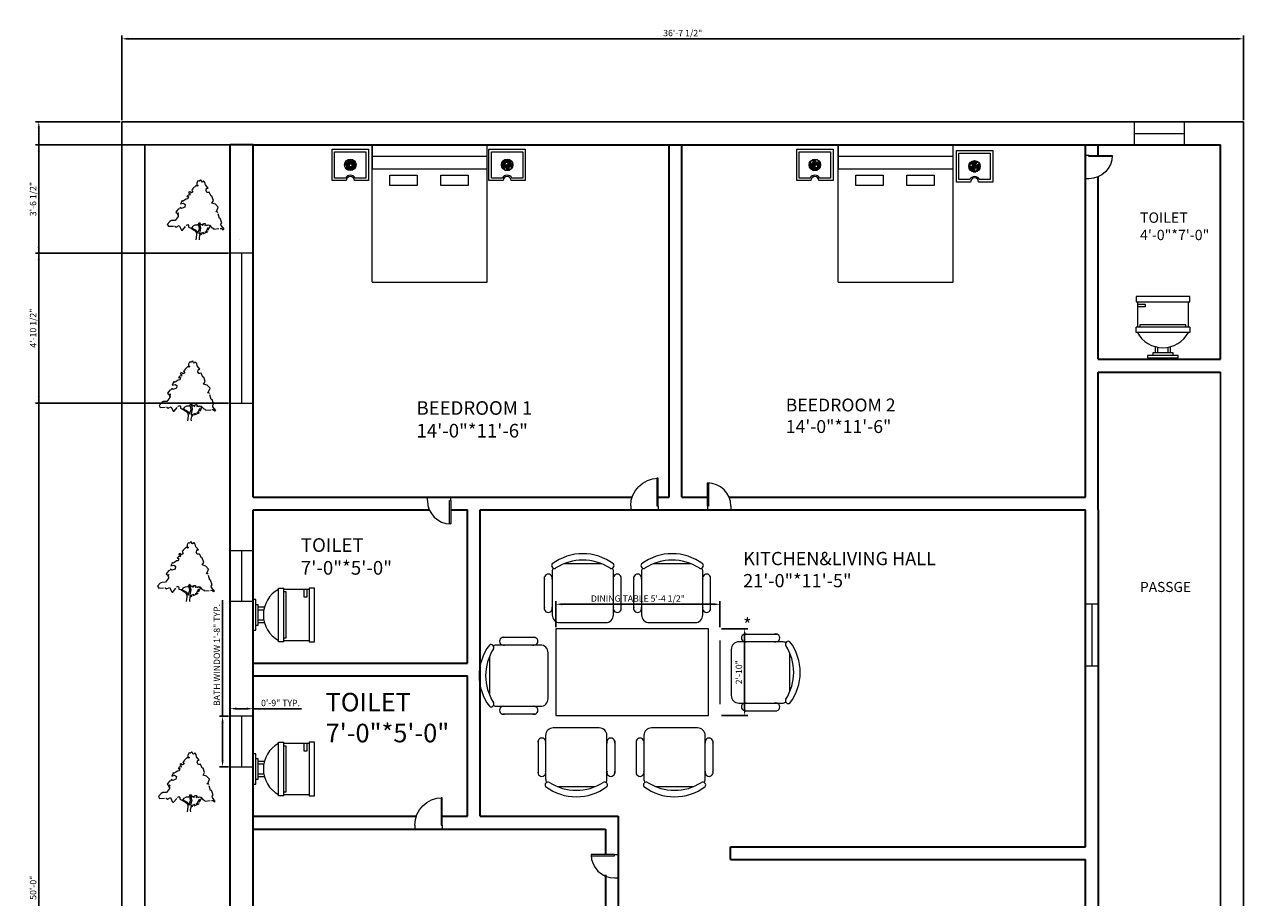
# Model space of a CAD drawing. Units: inches. Extents: x 2432 to 3786, y 1221 to 1905.
# Tile 2 of 4: x 2432 to 2910, y 1563 to 1905. Entities that reach past the tile are written whole.
import ezdxf

# ---------------------------------------------------------------- set-up
doc = ezdxf.new("R2010")
doc.units = ezdxf.units.IN
doc.linetypes.add('ACAD_ISO02W100', pattern=[15, 12, -3])
for name, color, linetype, lineweight, true_color in [('A-ANNO-DIMS', 32, 'Continuous', 18, 0xcd6928), ('A-AREA-IDEN', 244, 'Continuous', 18, 0x991b1e), ('A-FURN', 32, 'Continuous', 13, 0xcd6928), ('A-GLAZ', 116, 'Continuous', 18, 0x136734), ('A-WALL', 67, 'Continuous', 35, 0x727430), ('C-PROP', 67, 'Continuous', 25, 0x727430)]:
    doc.layers.add(name, color=color, linetype=linetype, lineweight=lineweight, true_color=true_color)
for name, color, linetype, lineweight in [('A-DOOR', 4, 'Continuous', 18), ('A-FLOR-FIXT', 9, 'Continuous', 18), ('L-PLNT', 3, 'ACAD_ISO02W100', 13)]:
    doc.layers.add(name, color=color, linetype=linetype, lineweight=lineweight)
doc.styles.get("Standard").update_dxf_attribs({"font": 'arial.ttf'})
doc.dimstyles.new('ISO-25', dxfattribs={"dimtxt": 2.5, "dimasz": 2.5, "dimexe": 1.25, "dimexo": 0.625, "dimtad": 1, "dimdec": 3, "dimlunit": 4, "dimtxsty": 'Standard', "dimcen": 2.5, "dimadec": 0, "dimazin": 0, "dimtfac": 1, "dimtdec": 3, "dimtmove": 0, "dimatfit": 3, "dimfxl": 1, "dimarcsym": 0})

# ---------------------------------------------------------------- blocks, each defined once
blk = doc.blocks.new('*U4')
for points in [[(22.0124, 137.721), (18.5475, 141.5624), (15.5282, 138.2446), (13.8028, 139.3505), (13.3714, 142.1153), (11.2148, 143.2214), (8.1954, 140.4564), (4.7447, 141.0094), (2.1567, 136.0326), (2.1567, 131.6088), (5.6074, 129.9499), (3.0193, 128.2909), (0.4313, 130.5029), (-6.9015, 123.3141), (-6.9015, 121.6552), (-9.9208, 119.9963), (-9.0581, 118.3373), (-6.9015, 115.0195), (-10.7835, 112.2546), (-14.6656, 115.0195), (-16.8222, 114.4665), (-17.6849, 112.2546), (-14.6656, 111.7016), (-14.2342, 107.2778), (-17.6065, 107.8307), (-21.5669, 103.9599), (-17.2536, 103.4069), (-18.9789, 97.8771), (-22.8609, 97.3241), (-27.1743, 94.5593), (-32.3504, 91.7944), (-32.7817, 94.0063), (-36.6638, 85.7116), (-29.7624, 87.3705), (-25.449, 84.6056), (-26.743, 77.9699), (-34.507, 75.205), (-37.9578, 77.4169), (-39.2518, 74.099), (-42.2711, 73.5461), (-44.8592, 70.2282), (-47.8786, 66.3574), (-43.9965, 63.0395), (-41.4085, 64.6985), (-44.3346, 59.8898), (-42.2089, 60.1377), (-42.5159, 55.7849), (-49.6039, 46.4502), (-58.2307, 45.8972), (-62.1127, 43.6853), (-68.5828, 36.4966), (-65.9947, 32.0727), (-50.0352, 32.6257), (-47.0159, 30.4138), (-39.6831, 33.7317), (-34.507, 22.6721), (-32.3504, 22.6721), (-22.4296, 34.8376), (-19.4102, 36.4966), (-17.2536, 33.7317), (-17.2536, 29.8608), (-13.8028, 28.7549), (-9.0581, 28.7549), (-7.3328, 32.6257), (-1.7254, 35.3906), (3.8821, 35.9436), (6.4701, 38.1555), (6.9014, 38.7085), (8.1954, 41.4734), (9.9208, 40.3674), (11.2148, 35.9436), (14.2341, 37.6025), (15.0968, 36.4966), (15.9595, 33.7317), (18.9789, 38.7085), (21.9982, 38.7085), (23.2922, 36.4966), (21.9982, 34.2847), (25.4489, 35.3906), (26.743, 33.7317), (29.7623, 35.9436), (32.7817, 34.8376), (38.8204, 28.7549), (41.4084, 27.6489), (43.5651, 25.437), (61.6813, 27.0959), (65.132, 23.7781), (67.7201, 24.884), (60.8186, 33.7317), (60.3873, 37.0495), (62.544, 40.3674), (58.662, 50.874), (56.5053, 50.874), (52.1919, 66.3574), (47.8785, 66.9103), (50.4665, 69.1222), (53.9172, 77.9699), (47.0158, 85.1586), (38.3891, 87.9235), (42.2711, 94.0063)], [(42.2711, 94.0063), (38.8204, 104.5129), (36.6637, 104.5129), (32.3503, 113.9135), (29.7623, 113.3605), (26.743, 113.3605), (24.5862, 117.7844), (25.8802, 123.8671), (29.331, 123.8671), (22.8609, 131.6088), (21.9982, 137.6916)], [(-9.9208, 28.2019), (0, 23.2251), (3.4507, 19.9072), (4.7447, 15.4834), (8.6267, 27.0959), (6.4701, 37.6025)], [(34.5071, 33.1787), (27.1743, 18.2483), (9.0581, 10.5066), (7.7641, 3.8708), (8.1954, 0)], [(8.1954, 40.3674), (11.2148, 27.6489), (8.1954, 13.8245), (24.5862, 19.9072), (32.7817, 34.2847)], [(-12.9401, 28.7549), (-2.588, 22.1191), (0.8626, 17.6953), (1.7253, 11.6125), (0, 0)]]:
    blk.add_lwpolyline(points)
blk = doc.blocks.new('FC15X27A')
for p, q in [((7.53125, 0), (-7.53125, 0)), ((-7.53125, 0), (-7.53125, -26.5)), ((7.53125, -26.5), (7.53125, 0)), ((-7.53125, -26.5), (7.53125, -26.5)), ((-5.53125, -28.5), (5.53125, -28.5))]:
    blk.add_line(p, q)
blk = doc.blocks.new('CHAIR7')
for p, q in [((5.12, 15.04), (17.88, 15.04)), ((20, 12), (3, 12)), ((0, 9), (0, -9)), ((23, -7.44), (23, 7.44)), ((3, -12), (20, -12)), ((5.12, -15), (17.88, -15))]:
    blk.add_line(p, q)
for centre, radius, start, end in [((5.56, 13.54), 1.56, 73.7398, 286.2602), ((17.44, 13.54), 1.56, 253.7398, 106.2602), ((3, 9), 3, 90, 180), ((20, 9), 3, 62.4156, 90), ((22.34, 11.12), 1.1, 53.3099, 212.0274), ((4.82, 0), 19.64, 327.5758, 32.4242), ((7, 0), 20, 323.1301, 36.8699), ((3, -9), 3, 180, 270), ((5.56, -13.5), 1.56, 73.7398, 286.2602), ((17.44, -13.5), 1.56, 253.7398, 106.2602), ((20, -9), 3, 270, 297.5844), ((22.34, -11.12), 1.1, 147.9726, 306.6901)]:
    blk.add_arc(centre, radius, start, end)
blk = doc.blocks.new('*U9')
for p, q in [((0, 0), (0, -6)), ((40, 0), (40, -6))]:
    blk.add_line(p, q)
blk.add_lwpolyline([(0, 0), (0, 40), (1.75, 40), (1.75, 0)], close=True)
blk.add_arc((0, 0), 40, 0, 90)
blk = doc.blocks.new('*U10')
for p, q in [((0, 0), (0, -6)), ((-40, 0), (-40, -6))]:
    blk.add_line(p, q)
blk.add_lwpolyline([(0, 0), (0, 40), (-1.75, 40), (-1.75, 0)], close=True)
blk.add_arc((0, 0), 40, 90, 180)
blk = doc.blocks.new('*U12')
for p, q in [((-10, 22), (-10, 12)), ((-10, 21), (-7, 21)), ((-7, 20), (-10, 20)), ((-7, 21), (-7, 20)), ((10, 12), (10, 22)), ((10.5, 12), (-10.5, 12)), ((-10.5, 10), (-10.5, 12)), ((10.5, 10), (-10.5, 10)), ((9, 13), (-9, 13)), ((-9, 13), (-9, 12)), ((9, 12), (9, 13)), ((10.5, 12), (10.5, 10)), ((4, 2), (-4, 2)), ((-4, 2), (-4, 1)), ((-3, 4.4065), (-3, 2)), ((-2, 2), (-2, 4.1658)), ((2, 4.1658), (2, 2)), ((3, 2), (3, 4.4065)), ((4, 1), (4, 2))]:
    blk.add_line(p, q)
for points in [[(10.5, 22), (10.5, 24), (-10.5, 24), (-10.5, 22)], [(6, 0), (6, 1), (-6, 1), (-6, 0)]]:
    blk.add_lwpolyline(points, close=True)
blk.add_arc((0, 15.3333), 11.3333, 208.0725, 331.9275)
blk = doc.blocks.new('BED-PLAN')
for p, q in [((0, 0), (0, 53.81)), ((0, 53.81), (0, 44.48)), ((45.03, 0), (45.03, 53.81)), ((45.03, 49.29), (0, 49.29)), ((0, 44.48), (45.03, 44.48)), ((0, 0), (45.03, 0))]:
    blk.add_line(p, q)
for points in [[(6.96, 41.97), (17.65, 41.97), (17.65, 37.91), (6.96, 37.91)], [(26.95, 41.97), (37.64, 41.97), (37.64, 37.91), (26.95, 37.91)]]:
    blk.add_lwpolyline(points, close=True)
blk = doc.blocks.new('BEDSIDE-TABLE')
h = blk.add_hatch()
h.set_pattern_fill('HOUND', color=256, scale=0.22)
h.set_pattern_definition([(0, (-2552.733, -1844.264), (1.397, 0.34925), [5.588, -2.794]), (90, (-2552.733, -1844.264), (-0.34925, -1.397), [5.588, -2.794])])
h.paths.add_polyline_path([(4.88, 6.16, 1), (9.38, 6.16, 1)])
for points in [[(5.54, 0), (0, 0), (0, 12.32), (14.26, 12.32), (14.26, 0), (8.72, 0)], [(5.25, 1), (1, 1), (1, 11.32), (13.26, 11.32), (13.26, 1), (9, 1)]]:
    blk.add_lwpolyline(points)
blk.add_circle((7.13, 6.16), 2.25)
for radius, start, end in [(2.13, 28.0704, 151.9296), (1.59, 0, 180)]:
    blk.add_arc((7.13, 0), radius, start, end)
blk = doc.blocks.new('WIN-BATH-20')
for p, q in [((9, 19.79), (0, 19.79)), ((0, 19.79), (0, 0)), ((9, 19.79), (4.5, 19.79)), ((4.5, 19.79), (4.5, 0)), ((9, 0), (9, 19.79)), ((0, 0), (9, 0))]:
    blk.add_line(p, q)
blk = doc.blocks.new('*D29')
at = {"layer": 'A-ANNO-DIMS', "color": 0, "lineweight": -2, "transparency": 16777216}
for p, q in [((2509.83, 1634.42), (2509.83, 1679.88)), ((2512.17, 1634.42), (2508.58, 1634.42)), ((2509.83, 1617.13), (2509.83, 1631.92)), ((2512.17, 1614.63), (2508.58, 1614.63))]:
    blk.add_line(p, q, dxfattribs=at)
at = {"layer": 'A-ANNO-DIMS', "color": 0, "lineweight": 5, "transparency": 16777216}
for points in [[(2509.41, 1631.92), (2510.24, 1631.92), (2509.83, 1634.42)], [(2509.41, 1617.13), (2510.24, 1617.13), (2509.83, 1614.63)]]:
    blk.add_solid(points, dxfattribs=at)
at = {"layer": 'Defpoints', "color": 0, "lineweight": 5, "transparency": 16777216}
for p in [(2509.83, 1634.42), (2512.8, 1634.42), (2512.8, 1614.63)]:
    blk.add_point(p, dxfattribs=at)
at = {"layer": 'A-ANNO-DIMS', "color": 0, "transparency": 16777216, "insert": (2507.91, 1658.4), "char_height": 2.5, "attachment_point": 5, "rotation": 90}
blk.add_mtext('BATH WINDOW 1\'-8" TYP.', dxfattribs=at)
blk = doc.blocks.new('*D30')
at = {"layer": 'A-ANNO-DIMS', "color": 0, "lineweight": -2, "transparency": 16777216}
for p, q in [((2512.8, 1635.05), (2512.8, 1638.64)), ((2521.8, 1635.05), (2521.8, 1638.64)), ((2515.3, 1637.39), (2519.3, 1637.39)), ((2521.8, 1637.39), (2540.79, 1637.39))]:
    blk.add_line(p, q, dxfattribs=at)
at = {"layer": 'A-ANNO-DIMS', "color": 0, "lineweight": 5, "transparency": 16777216}
for points in [[(2515.3, 1637.81), (2515.3, 1636.97), (2512.8, 1637.39)], [(2519.3, 1637.81), (2519.3, 1636.97), (2521.8, 1637.39)]]:
    blk.add_solid(points, dxfattribs=at)
at = {"layer": 'Defpoints', "color": 0, "lineweight": 5, "transparency": 16777216}
for p in [(2512.8, 1634.42), (2521.8, 1637.39), (2521.8, 1634.42)]:
    blk.add_point(p, dxfattribs=at)
at = {"layer": 'A-ANNO-DIMS', "color": 0, "transparency": 16777216, "insert": (2532.54, 1639.29), "char_height": 2.5, "attachment_point": 5}
blk.add_mtext('0\'-9" TYP.', dxfattribs=at)
blk = doc.blocks.new('*D33')
at = {"layer": 'A-ANNO-DIMS', "color": 0, "lineweight": -2, "transparency": 16777216}
for p, q in [((2640.37, 1669.27), (2640.37, 1679.54)), ((2702.18, 1678.29), (2642.87, 1678.29)), ((2704.68, 1669.27), (2704.68, 1679.54))]:
    blk.add_line(p, q, dxfattribs=at)
at = {"layer": 'A-ANNO-DIMS', "color": 0, "lineweight": 5, "transparency": 16777216}
for points in [[(2642.87, 1678.71), (2642.87, 1677.88), (2640.37, 1678.29)], [(2702.18, 1678.71), (2702.18, 1677.88), (2704.68, 1678.29)]]:
    blk.add_solid(points, dxfattribs=at)
at = {"layer": 'Defpoints', "color": 0, "lineweight": 5, "transparency": 16777216}
for p in [(2640.37, 1678.29), (2640.37, 1668.65), (2704.68, 1668.65)]:
    blk.add_point(p, dxfattribs=at)
at = {"layer": 'A-ANNO-DIMS', "color": 0, "transparency": 16777216, "insert": (2672.53, 1680.21), "char_height": 2.5, "attachment_point": 5}
blk.add_mtext('DINING TABLE 5\'-4 1/2"', dxfattribs=at)
blk = doc.blocks.new('*D34')
at = {"layer": 'A-ANNO-DIMS', "color": 0, "lineweight": -2, "transparency": 16777216}
for p, q in [((2705.31, 1668.65), (2715.58, 1668.65)), ((2714.33, 1637.16), (2714.33, 1666.15)), ((2705.31, 1634.66), (2715.58, 1634.66))]:
    blk.add_line(p, q, dxfattribs=at)
at = {"layer": 'A-ANNO-DIMS', "color": 0, "lineweight": 5, "transparency": 16777216}
for points in [[(2713.92, 1666.15), (2714.75, 1666.15), (2714.33, 1668.65)], [(2713.92, 1637.16), (2714.75, 1637.16), (2714.33, 1634.66)]]:
    blk.add_solid(points, dxfattribs=at)
at = {"layer": 'Defpoints', "color": 0, "lineweight": 5, "transparency": 16777216}
for p in [(2704.68, 1668.65), (2714.33, 1668.65), (2704.68, 1634.66)]:
    blk.add_point(p, dxfattribs=at)
at = {"layer": 'A-ANNO-DIMS', "color": 0, "transparency": 16777216, "insert": (2712.43, 1651.65), "char_height": 2.5, "attachment_point": 5, "rotation": 90}
blk.add_mtext('2\'-10"', dxfattribs=at)
blk = doc.blocks.new('*D35')
at = {"layer": 'A-ANNO-DIMS', "color": 0, "lineweight": -2, "transparency": 16777216}
for p, q in [((2470.39, 1867.88), (2470.39, 1901.05)), ((2909.8, 1867.88), (2909.8, 1901.05)), ((2472.89, 1899.8), (2907.3, 1899.8))]:
    blk.add_line(p, q, dxfattribs=at)
at = {"layer": 'A-ANNO-DIMS', "color": 0, "lineweight": 5, "transparency": 16777216}
for points in [[(2472.89, 1900.22), (2472.89, 1899.38), (2470.39, 1899.8)], [(2907.3, 1900.22), (2907.3, 1899.38), (2909.8, 1899.8)]]:
    blk.add_solid(points, dxfattribs=at)
at = {"layer": 'Defpoints', "color": 0, "lineweight": 5, "transparency": 16777216}
for p in [(2909.8, 1899.8), (2470.39, 1867.25), (2909.8, 1867.25)]:
    blk.add_point(p, dxfattribs=at)
at = {"layer": 'A-ANNO-DIMS', "color": 0, "transparency": 16777216, "insert": (2690.09, 1901.72), "char_height": 2.5, "attachment_point": 5}
blk.add_mtext('36\'-7 1/2"', dxfattribs=at)
blk = doc.blocks.new('*D36')
at = {"layer": 'A-ANNO-DIMS', "color": 0, "lineweight": -2, "transparency": 16777216}
for p, q in [((2469.77, 1867.25), (2436.59, 1867.25)), ((2437.84, 1269.75), (2437.84, 1864.75)), ((2469.77, 1267.25), (2436.59, 1267.25))]:
    blk.add_line(p, q, dxfattribs=at)
at = {"layer": 'A-ANNO-DIMS', "color": 0, "lineweight": 5, "transparency": 16777216}
for points in [[(2437.42, 1864.75), (2438.26, 1864.75), (2437.84, 1867.25)], [(2437.42, 1269.75), (2438.26, 1269.75), (2437.84, 1267.25)]]:
    blk.add_solid(points, dxfattribs=at)
at = {"layer": 'Defpoints', "color": 0, "lineweight": 5, "transparency": 16777216}
for p in [(2437.84, 1867.25), (2470.39, 1867.25), (2470.39, 1267.25)]:
    blk.add_point(p, dxfattribs=at)
at = {"layer": 'A-ANNO-DIMS', "color": 0, "transparency": 16777216, "insert": (2435.94, 1567.25), "char_height": 2.5, "attachment_point": 5, "rotation": 90}
blk.add_mtext('50\'-0"', dxfattribs=at)
blk = doc.blocks.new('*D43')
at = {"layer": 'A-ANNO-DIMS', "color": 0, "lineweight": -2, "transparency": 16777216}
for p, q in [((2512.17, 1858.25), (2436.59, 1858.25)), ((2437.84, 1818.28), (2437.84, 1855.75)), ((2512.17, 1815.78), (2436.59, 1815.78))]:
    blk.add_line(p, q, dxfattribs=at)
at = {"layer": 'A-ANNO-DIMS', "color": 0, "lineweight": 5, "transparency": 16777216}
for points in [[(2437.42, 1855.75), (2438.26, 1855.75), (2437.84, 1858.25)], [(2437.42, 1818.28), (2438.26, 1818.28), (2437.84, 1815.78)]]:
    blk.add_solid(points, dxfattribs=at)
at = {"layer": 'Defpoints', "color": 0, "lineweight": 5, "transparency": 16777216}
for p in [(2437.84, 1858.25), (2512.8, 1858.25), (2512.8, 1815.78)]:
    blk.add_point(p, dxfattribs=at)
at = {"layer": 'A-ANNO-DIMS', "color": 0, "transparency": 16777216, "insert": (2435.92, 1837.02), "char_height": 2.5, "attachment_point": 5, "rotation": 90}
blk.add_mtext('3\'-6 1/2"', dxfattribs=at)
blk = doc.blocks.new('*D44')
at = {"layer": 'A-ANNO-DIMS', "color": 0, "lineweight": -2, "transparency": 16777216}
for p, q in [((2512.17, 1815.78), (2436.59, 1815.78)), ((2437.84, 1759.63), (2437.84, 1813.28)), ((2512.17, 1757.13), (2436.59, 1757.13))]:
    blk.add_line(p, q, dxfattribs=at)
at = {"layer": 'A-ANNO-DIMS', "color": 0, "lineweight": 5, "transparency": 16777216}
for points in [[(2437.42, 1813.28), (2438.26, 1813.28), (2437.84, 1815.78)], [(2437.42, 1759.63), (2438.26, 1759.63), (2437.84, 1757.13)]]:
    blk.add_solid(points, dxfattribs=at)
at = {"layer": 'Defpoints', "color": 0, "lineweight": 5, "transparency": 16777216}
for p in [(2437.84, 1815.78), (2512.8, 1815.78), (2512.8, 1757.13)]:
    blk.add_point(p, dxfattribs=at)
at = {"layer": 'A-ANNO-DIMS', "color": 0, "transparency": 16777216, "insert": (2435.92, 1786.45), "char_height": 2.5, "attachment_point": 5, "rotation": 90}
blk.add_mtext('4\'-10 1/2"', dxfattribs=at)

msp = doc.modelspace()

# ---------------------------------------------------------------- linework, layer by layer
at = {"layer": 'A-FURN'}
msp.add_line((2613.457, 1848.9224), (2613.457, 1853.7325), dxfattribs=at)
at = {"layer": 'A-GLAZ'}
for p, q in [((2516.3906, 1821.1517), (2516.3906, 1821.1517)), ((2521.7964, 1815.7822), (2512.7964, 1815.7822)), ((2512.7964, 1815.7822), (2512.7964, 1757.1277)), ((2521.7964, 1815.7822), (2517.2964, 1815.7822)), ((2517.2964, 1815.7822), (2517.2964, 1757.1277)), ((2521.7964, 1757.1277), (2521.7964, 1815.7822)), ((2512.7964, 1757.1277), (2521.7964, 1757.1277)), ((2521.7964, 1699.2785), (2521.7964, 1699.2785)), ((2852.7964, 1678.2982), (2847.7964, 1678.2982)), ((2847.7964, 1678.2982), (2847.7964, 1654.1432)), ((2852.7964, 1678.2982), (2850.2964, 1678.2982)), ((2850.2964, 1678.2982), (2850.2964, 1654.1432)), ((2852.7964, 1654.1432), (2852.7964, 1678.2982)), ((2847.7964, 1654.1432), (2852.7964, 1654.1432))]:
    msp.add_line(p, q, dxfattribs=at)
at = {"layer": 'A-WALL'}
for p, q in [((2512.7964, 1699.2785), (2512.7964, 1858.2516)), ((2521.7964, 1858.2516), (2512.7964, 1858.2516)), ((2521.7964, 1720.2516), (2521.7964, 1858.2516)), ((2521.7964, 1858.2516), (2689.7964, 1858.2516)), ((2684.7964, 1720.2516), (2684.7964, 1858.2516)), ((2689.7964, 1720.2516), (2689.7964, 1858.2516)), ((2689.7964, 1858.2516), (2852.7964, 1858.2516)), ((2847.7964, 1720.2516), (2847.7964, 1858.2516)), ((2852.7964, 1858.2516), (2900.7964, 1858.2516)), ((2852.7964, 1854.1131), (2852.7964, 1858.2516)), ((2900.7964, 1774.2516), (2900.7964, 1858.2516)), ((2852.7964, 1774.2516), (2852.7964, 1845.7452)), ((2852.7964, 1774.2516), (2900.7964, 1774.2516)), ((2852.7964, 1769.2516), (2900.7964, 1769.2516)), ((2852.7964, 1715.2516), (2852.7964, 1769.2516)), ((2521.7964, 1720.2516), (2670.2308, 1720.2516)), ((2680.4218, 1720.2516), (2684.7964, 1720.2516)), ((2689.7964, 1720.2516), (2699.8199, 1720.2516)), ((2708.213, 1720.2516), (2847.7964, 1720.2516)), ((2512.7964, 1276.2516), (2512.7964, 1715.2516)), ((2521.7964, 1715.2516), (2590.8232, 1715.2516)), ((2521.7964, 1276.2516), (2521.7964, 1715.2516)), ((2599.1801, 1715.2516), (2605.7964, 1715.2516)), ((2605.7964, 1655.2516), (2605.7964, 1715.2516)), ((2610.7964, 1595.2516), (2610.7964, 1715.2516)), ((2610.7964, 1715.2516), (2847.7964, 1715.2516)), ((2847.7964, 1583.2516), (2847.7964, 1715.2516)), ((2852.7964, 1715.2516), (2852.7964, 1422.2516)), ((2521.7964, 1655.2516), (2605.7964, 1655.2516)), ((2521.7964, 1650.2516), (2605.7964, 1650.2516)), ((2605.7964, 1595.2516), (2605.7964, 1650.2516)), ((2521.7964, 1595.2516), (2585.6142, 1595.2516)), ((2521.7964, 1595.2516), (2585.6142, 1595.2516)), ((2595.398, 1595.2516), (2605.7964, 1595.2516)), ((2595.398, 1595.2516), (2605.7964, 1595.2516)), ((2610.7964, 1595.2516), (2659.7964, 1595.2516)), ((2659.7964, 1595.2516), (2664.7964, 1595.2516)), ((2664.7964, 1595.2516), (2664.7964, 1588.5936)), ((2521.7964, 1590.2516), (2610.7964, 1590.2516)), ((2521.7964, 1590.2516), (2659.7964, 1590.2516)), ((2659.7964, 1590.2516), (2659.7964, 1580.2021)), ((2664.7964, 1590.2516), (2664.7964, 1470.2516)), ((2708.7964, 1583.2516), (2847.7964, 1583.2516)), ((2708.7964, 1578.2516), (2708.7964, 1583.2516)), ((2852.7964, 1583.2516), (2852.7964, 1578.2516)), ((2708.7964, 1578.2516), (2847.7964, 1578.2516)), ((2847.7964, 1422.2516), (2847.7964, 1578.2516)), ((2659.7964, 1572.3142), (2659.7964, 1470.2516))]:
    msp.add_line(p, q, dxfattribs=at)
at = {"layer": 'C-PROP'}
for p, q in [((2470.3906, 1867.2516), (2909.7964, 1867.2516)), ((2470.3906, 1267.2516), (2470.3906, 1867.2516)), ((2909.7964, 1267.2516), (2909.7964, 1867.2516)), ((2479.3906, 1858.2516), (2512.7964, 1858.2516)), ((2479.3906, 1276.2516), (2479.3906, 1858.2516)), ((2900.7964, 1276.2516), (2900.7964, 1769.2516))]:
    msp.add_line(p, q, dxfattribs=at)

# ---------------------------------------------------------------- block references
at = {"layer": 'A-DOOR', "yscale": 0.2277050421196423, "zscale": 0.2277050421196423}
for name, p, xscale, rotation in [('*U10', (2849.1996, 1854.1131), -0.2277050421196423, 270), ('*U9', (2599.1801, 1718.874), 0.2277050421196423, 180), ('*U10', (2663.3306, 1580.2021), 0.2277050421196423, 90.00000000000003)]:
    msp.add_blockref(name, p, dxfattribs=dict(at, xscale=xscale, rotation=rotation))
at = {"layer": 'A-DOOR'}
for p, xscale, yscale, zscale in [((2680.4218, 1716.8961), -0.2682308585481125, 0.2682308585481125, 0.2682308585481125), ((2699.8199, 1716.7139), 0.2277050421196423, 0.2277050421196423, 0.2277050421196423), ((2595.8674, 1591.7623), -0.2682308585481125, 0.2682308585481125, 0.2682308585481125)]:
    msp.add_blockref('*U9', p, dxfattribs=dict(at, xscale=xscale, yscale=yscale, zscale=zscale))
at = {"layer": 'A-FLOR-FIXT'}
msp.add_blockref('*U12', (2878.1721, 1774.7965), dxfattribs=at)
at = {"layer": 'A-FLOR-FIXT', "rotation": 270}
for p in [(2521.7964, 1674.1217), (2521.7964, 1613.7575)]:
    msp.add_blockref('*U12', p, dxfattribs=at)
at = {"layer": 'A-FURN'}
for name, p in [('BED-PLAN', (2568.4228, 1804.445)), ('BED-PLAN', (2750.933, 1804.445)), ('BEDSIDE-TABLE', (2552.733, 1844.264)), ('BEDSIDE-TABLE', (2614.1647, 1844.264)), ('BEDSIDE-TABLE', (2734.7336, 1844.264)), ('BEDSIDE-TABLE', (2797.2703, 1843.6867)), ('CHAIR7', (2709.0862, 1651.5871))]:
    msp.add_blockref(name, p, dxfattribs=at)
for p, rotation in [((2650.9497, 1671.101), 89.99999999999999), ((2685.9435, 1671.101), 89.99999999999999), ((2637.3343, 1650.3092), 180), ((2648.3909, 1629.8671), 270), ((2686.8767, 1629.8671), 270)]:
    msp.add_blockref('CHAIR7', p, dxfattribs=dict(at, rotation=rotation))
at = {"layer": 'A-FURN', "xscale": 2.256575257006187, "yscale": 2.256575257006187, "zscale": 2.256575257006187, "rotation": 90}
msp.add_blockref('FC15X27A', (2640.3725, 1651.651), dxfattribs=at)
at = {"layer": 'A-GLAZ', "rotation": 89.99999999999785}
msp.add_blockref('WIN-BATH-20', (2886.6909, 1858.2511), dxfattribs=at)
at = {"layer": 'A-GLAZ'}
for p in [(2512.796, 1679.4891), (2512.796, 1614.633)]:
    msp.add_blockref('WIN-BATH-20', p, dxfattribs=at)
at = {"layer": 'L-PLNT', "xscale": 0.163121370253731, "yscale": 0.163121370253731, "zscale": 0.163121370253731}
for p in [(2499.351, 1821.1076), (2496.1269, 1750.1904), (2495.5627, 1679.3707), (2495.917, 1597.0309)]:
    msp.add_blockref('*U4', p, dxfattribs=at)

# ---------------------------------------------------------------- texts
at = {"layer": 'A-AREA-IDEN', "attachment_point": 1}
for s, width, gutter_width, insert, char_height in [('TOILET\\P4\'-0"*7\'-0"', 38.389911, 20.3643, (2869.2205, 1831.7864), 4.072854), ('BEEDROOM 1\\P14\'-0"*11\'-6"', 212.266575, 26.6785, (2585.8015, 1757.8441), 5.335702), ('BEEDROOM 2\\P14\'-0"*11\'-6"', 192.266446, 25.2979, (2730.4381, 1758.8716), 5.059577), ('TOILET\\P7\'-0"*5\'-0"', 136.360909, 26.8012, (2540.4969, 1704.1721), 5.360246), ('KITCHEN&LIVING HALL\\P21\'-0"*11\'-5"\\P\\P*', 215.514927, 25.9597, (2713.7583, 1698.7933), 5.191942), ('PASSGE', 49.88256, 19.7443, (2869.216, 1687.0332), 3.94885), ('TOILET\\P7\'-0"*5\'-0"', 184.784121, 36.3186, (2550.2029, 1643.5803), 7.263726)]:
    msp.add_mtext_dynamic_manual_height_columns(s, width=width, gutter_width=gutter_width, heights=[0], dxfattribs=dict(at, insert=insert, char_height=char_height))

# ---------------------------------------------------------------- dimensions: what is measured, and where the dimension line sits
at = {"layer": 'A-ANNO-DIMS'}
dim = msp.add_linear_dim(base=(2909.7964, 1899.8016), p1=(2470.3906, 1867.2516), p2=(2909.7964, 1867.2516), dimstyle='ISO-25', override={"dimdec": 1, "dimlfac": 1, "dimrnd": 0, "dimzin": 1, "dimdsep": 46, "dimlunit": 4, "dimfrac": 2}, dxfattribs=at)
dim.commit()
dim.dimension.update_dxf_attribs({"geometry": '*D35', "text_midpoint": (2690.0935, 1901.7201)})
for base, p1, p2, picture, middle in [((2437.8406, 1867.2516), (2470.3906, 1267.2516), (2470.3906, 1867.2516), '*D36', (2435.9391, 1567.2516)), ((2437.8406, 1858.2516), (2512.7964, 1815.7822), (2512.7964, 1858.2516), '*D43', (2435.9221, 1837.0169)), ((2437.8406, 1815.7822), (2512.7964, 1757.1277), (2512.7964, 1815.7822), '*D44', (2435.9229, 1786.455)), ((2714.3318, 1668.6458), (2704.6849, 1634.6562), (2704.6849, 1668.6458), '*D34', (2712.4304, 1651.651))]:
    dim = msp.add_linear_dim(base=base, p1=p1, p2=p2, angle=90, dimstyle='ISO-25', override={"dimdec": 1, "dimlfac": 1, "dimrnd": 0, "dimzin": 1, "dimdsep": 46, "dimlunit": 4, "dimfrac": 2}, dxfattribs=at)
    dim.commit()
    dim.dimension.update_dxf_attribs({"geometry": picture, "text_midpoint": middle})
for base, p1, p2, angle, text, picture, middle in [((2640.3725, 1678.2927), (2704.6849, 1668.6458), (2640.3725, 1668.6458), 180, 'DINING TABLE <>', '*D33', (2672.5287, 1680.2103)), ((2509.828, 1634.4224), (2512.7964, 1614.6326), (2512.7964, 1634.4224), 90, 'BATH WINDOW <> TYP.', '*D29', (2507.9095, 1658.4009))]:
    dim = msp.add_linear_dim(base=base, p1=p1, p2=p2, angle=angle, text=text, dimstyle='ISO-25', override={"dimdec": 1, "dimlfac": 1, "dimrnd": 0, "dimzin": 1, "dimdsep": 46, "dimlunit": 4, "dimfrac": 2}, dxfattribs=at)
    dim.commit()
    dim.dimension.update_dxf_attribs({"geometry": picture, "text_midpoint": middle})
dim = msp.add_linear_dim(base=(2521.7964, 1637.3909), p1=(2512.7964, 1634.4224), p2=(2521.7964, 1634.4224), text='<> TYP.', dimstyle='ISO-25', override={"dimdec": 1, "dimlfac": 1, "dimrnd": 0, "dimzin": 1, "dimdsep": 46, "dimlunit": 4, "dimfrac": 2}, dxfattribs=at)
dim.commit()
dim.dimension.update_dxf_attribs({"geometry": '*D30', "text_midpoint": (2532.5408, 1639.2923)})

doc.saveas('drawing.dxf')
